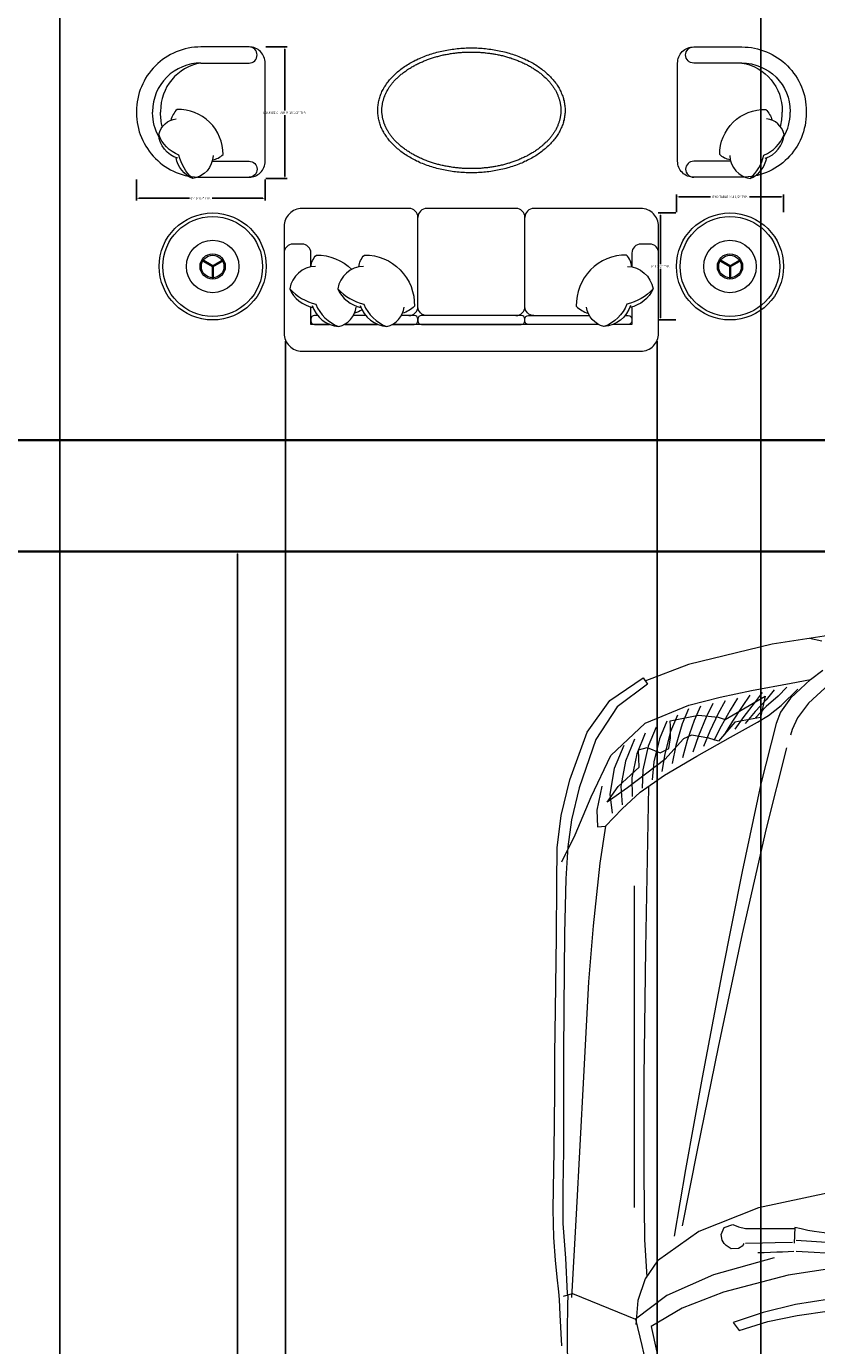
# Model space of a CAD drawing. Units: inches. Extents: x -36 to 401, y -686 to 73.
# Tile 7 of 15: x 184 to 248, y -485 to -379. Entities that reach past the tile are written whole.
import ezdxf

# ---------------------------------------------------------------- set-up
doc = ezdxf.new("R2010")
doc.units = ezdxf.units.IN
doc.header["$MEASUREMENT"] = 0
for name, color, linetype, lineweight in [('A-ANNO-DIMS', 2, 'Continuous', 18), ('A-FURN', 8, 'Continuous', 13), ('A-WALL', 7, 'Continuous', 35), ('C-PKNG-VEHI', 8, 'Continuous', 13)]:
    doc.layers.add(name, color=color, linetype=linetype, lineweight=lineweight)
doc.styles.get("Standard").update_dxf_attribs({"font": 'arial.ttf'})
doc.dimstyles.get("Standard").update_dxf_attribs({"dimtxt": 0.18, "dimasz": 0.18, "dimexe": 0.18, "dimexo": 0.0625, "dimgap": 0.09, "dimtad": 0, "dimtih": 1, "dimtoh": 1, "dimdec": 0, "dimzin": 0, "dimdsep": 46, "dimlunit": 3, "dimtxsty": 'Standard', "dimcen": 0.09, "dimadec": 0, "dimazin": 0, "dimtfac": 1, "dimtdec": 0, "dimtofl": 0, "dimtmove": 0, "dimatfit": 3, "dimfxl": 1, "dimtolj": 1, "dimtzin": 0, "dimarcsym": 0})

# ---------------------------------------------------------------- blocks, each defined once
blk = doc.blocks.new('*D3')
at = {"layer": 'A-ANNO-DIMS', "color": 0, "lineweight": -2, "transparency": 16777216}
for p, q in [((200.9, -421.21), (201.62, -421.21)), ((201.44, -421.39), (201.44, -532.06)), ((201.44, -649.03), (201.44, -538.36)), ((200.9, -649.21), (201.62, -649.21))]:
    blk.add_line(p, q, dxfattribs=at)
at = {"layer": 'A-ANNO-DIMS', "color": 0, "transparency": 16777216}
for points in [[(201.41, -421.39), (201.47, -421.39), (201.44, -421.21)], [(201.41, -649.03), (201.47, -649.03), (201.44, -649.21)]]:
    blk.add_solid(points, dxfattribs=at)
at = {"layer": 'Defpoints', "color": 0, "transparency": 16777216}
for p in [(200.84, -421.21), (200.84, -649.21), (201.44, -649.21)]:
    blk.add_point(p, dxfattribs=at)
at = {"layer": 'A-ANNO-DIMS', "color": 0, "transparency": 16777216, "insert": (201.44, -535.21), "char_height": 6, "attachment_point": 5}
blk.add_mtext("\\A1;19'", dxfattribs=at)
blk = doc.blocks.new('CHAIR-LOUNGE')
at = {"ltscale": 0.03}
blk.add_lwpolyline([(10.39, 5.37), (10.39, 9.33, 0.414214), (9.09, 10.63), (5.2, 10.63, 0.414214), (0, 5.43), (0, 5.37), (0, 5.3, 0.414214), (5.2, 0.11), (9.09, 0.11, 0.414214), (10.39, 1.4), (10.39, 5.37)], format="xyb", dxfattribs=at)
for points in [[(5.2, 9.33), (9.09, 9.33, 0.414214), (9.74, 9.98), (9.74, 9.98, 0.414214), (9.09, 10.63)], [(5.2, 9.33, 0.414214), (1.3, 5.43), (1.3, 5.37)], [(5.2, 9.33, 0.372719), (1.95, 5.43), (1.95, 5.37)], [(1.81, 3.37, -0.130591), (1.3, 5.3), (1.3, 5.37)], [(2.09, 4.19, -0.072384), (1.95, 5.3), (1.95, 5.37)], [(6.14, 1.53, 0.165541), (6.99, 1.94, 0.425989), (3.27, 5.58, 0.121523), (2.76, 4.72, -7.115464)], [(3.33, 1.64, -0.306663), (1.79, 3.57, -0.30633), (3.2, 4.84, 0.872847)], [(4.54, 0, -0.14773), (3.42, 1.9, -0.213343), (1.79, 3.57, -0.178662)], [(6.18, 1.86, -0.356772), (4.54, 0, -0.249542), (3.19, 1.69, 9.61688)], [(6.11, 1.4), (9.09, 1.4, -0.414214), (9.74, 0.76), (9.74, 0.76, -0.414214), (9.09, 0.11)]]:
    blk.add_lwpolyline(points, format="xyb")
blk = doc.blocks.new('END-TABLE-ROUND')
at = {"ltscale": 0.03}
for p, q in [((4.3, 4.28), (3.42, 4.79)), ((4.34, 4.36), (3.46, 4.87)), ((4.28, 4.32), (4.28, 3.31)), ((4.3, 4.36), (5.18, 4.87)), ((4.34, 4.28), (5.22, 4.79)), ((4.37, 4.32), (4.37, 3.31))]:
    blk.add_line(p, q, dxfattribs=at)
for radius in [4.32, 2.12, 1.02, 0.911]:
    blk.add_circle((4.32, 4.32), radius, dxfattribs=at)
blk.add_circle((4.32, 4.32), 4.03)
blk = doc.blocks.new('*D49')
at = {"layer": 'A-ANNO-DIMS', "color": 0, "lineweight": -2, "transparency": 16777216}
for p, q in [((203.74, -380.47), (205.45, -380.47)), ((205.27, -380.65), (205.27, -385.6)), ((205.27, -390.92), (205.27, -385.97)), ((203.74, -391.1), (205.45, -391.1))]:
    blk.add_line(p, q, dxfattribs=at)
at = {"layer": 'A-ANNO-DIMS', "color": 0, "transparency": 16777216}
for points in [[(205.24, -380.65), (205.3, -380.65), (205.27, -380.47)], [(205.24, -390.92), (205.3, -390.92), (205.27, -391.1)]]:
    blk.add_solid(points, dxfattribs=at)
at = {"layer": 'Defpoints', "color": 0, "transparency": 16777216}
for p in [(203.68, -380.47), (205.27, -380.47), (203.68, -391.1)]:
    blk.add_point(p, dxfattribs=at)
at = {"layer": 'A-ANNO-DIMS', "color": 0, "transparency": 16777216, "insert": (205.27, -385.78), "char_height": 0.18, "attachment_point": 5}
blk.add_mtext('\\A1;LOUNGE CHAIR 0\'-10 1/2" TYP.', dxfattribs=at)
blk = doc.blocks.new('*D50')
at = {"layer": 'A-ANNO-DIMS', "color": 0, "lineweight": -2, "transparency": 16777216}
for p, q in [((193.29, -391.16), (193.29, -392.87)), ((203.68, -391.16), (203.68, -392.87)), ((193.47, -392.69), (197.56, -392.69)), ((203.5, -392.69), (199.4, -392.69))]:
    blk.add_line(p, q, dxfattribs=at)
at = {"layer": 'A-ANNO-DIMS', "color": 0, "transparency": 16777216}
for points in [[(193.47, -392.66), (193.47, -392.72), (193.29, -392.69)], [(203.5, -392.66), (203.5, -392.72), (203.68, -392.69)]]:
    blk.add_solid(points, dxfattribs=at)
at = {"layer": 'Defpoints', "color": 0, "transparency": 16777216}
for p in [(193.29, -391.1), (203.68, -391.1), (203.68, -392.69)]:
    blk.add_point(p, dxfattribs=at)
at = {"layer": 'A-ANNO-DIMS', "color": 0, "transparency": 16777216, "insert": (198.48, -392.69), "char_height": 0.18, "attachment_point": 5}
blk.add_mtext('\\A1;0\'-10 1/2" TYP.', dxfattribs=at)
blk = doc.blocks.new('*D51')
at = {"layer": 'A-ANNO-DIMS', "color": 0, "lineweight": -2, "transparency": 16777216}
for p, q in [((236.89, -393.81), (236.89, -392.39)), ((237.07, -392.57), (239.64, -392.57)), ((245.36, -392.57), (242.79, -392.57)), ((245.54, -393.81), (245.54, -392.39))]:
    blk.add_line(p, q, dxfattribs=at)
at = {"layer": 'A-ANNO-DIMS', "color": 0, "transparency": 16777216}
for points in [[(237.07, -392.54), (237.07, -392.6), (236.89, -392.57)], [(245.36, -392.54), (245.36, -392.6), (245.54, -392.57)]]:
    blk.add_solid(points, dxfattribs=at)
at = {"layer": 'Defpoints', "color": 0, "transparency": 16777216}
for p in [(245.54, -392.57), (236.89, -393.87), (245.54, -393.87)]:
    blk.add_point(p, dxfattribs=at)
at = {"layer": 'A-ANNO-DIMS', "color": 0, "transparency": 16777216, "insert": (241.22, -392.57), "char_height": 0.18, "attachment_point": 5}
blk.add_mtext('\\A1;END TABLE 0\'-8 1/2" TYP.', dxfattribs=at)
blk = doc.blocks.new('*D52')
at = {"layer": 'A-ANNO-DIMS', "color": 0, "lineweight": -2, "transparency": 16777216}
for p, q in [((236.83, -393.87), (235.42, -393.87)), ((235.6, -394.05), (235.6, -398.01)), ((235.6, -402.33), (235.6, -398.37)), ((236.83, -402.51), (235.42, -402.51))]:
    blk.add_line(p, q, dxfattribs=at)
at = {"layer": 'A-ANNO-DIMS', "color": 0, "transparency": 16777216}
for points in [[(235.57, -394.05), (235.63, -394.05), (235.6, -393.87)], [(235.57, -402.33), (235.63, -402.33), (235.6, -402.51)]]:
    blk.add_solid(points, dxfattribs=at)
at = {"layer": 'Defpoints', "color": 0, "transparency": 16777216}
for p in [(235.6, -393.87), (236.89, -393.87), (236.89, -402.51)]:
    blk.add_point(p, dxfattribs=at)
at = {"layer": 'A-ANNO-DIMS', "color": 0, "transparency": 16777216, "insert": (235.6, -398.19), "char_height": 0.18, "attachment_point": 5}
blk.add_mtext('\\A1;0\'-8 1/2" TYP.', dxfattribs=at)
blk = doc.blocks.new('*D73')
at = {"layer": 'A-ANNO-DIMS', "color": 0, "lineweight": -2, "transparency": 16777216}
for p, q in [((177.19, -421.27), (177.19, -685.69)), ((253.69, -421.27), (253.69, -685.69)), ((177.37, -685.51), (214.9, -685.51)), ((253.51, -685.51), (215.98, -685.51))]:
    blk.add_line(p, q, dxfattribs=at)
at = {"layer": 'A-ANNO-DIMS', "color": 0, "transparency": 16777216}
for points in [[(177.37, -685.48), (177.37, -685.54), (177.19, -685.51)], [(253.51, -685.48), (253.51, -685.54), (253.69, -685.51)]]:
    blk.add_solid(points, dxfattribs=at)
at = {"layer": 'Defpoints', "color": 0, "transparency": 16777216}
for p in [(177.19, -421.21), (253.69, -421.21), (253.69, -685.51)]:
    blk.add_point(p, dxfattribs=at)
at = {"layer": 'A-ANNO-DIMS', "color": 0, "transparency": 16777216, "insert": (215.44, -685.51), "char_height": 0.18, "attachment_point": 5}
blk.add_mtext('\\A1;6\'-4 1/2"', dxfattribs=at)
blk = doc.blocks.new('*D87')
at = {"layer": 'A-ANNO-DIMS', "color": 0, "lineweight": -2, "transparency": 16777216}
for p, q in [((243.7, -154.81), (243.7, -685.69)), ((187.11, -163.6), (187.11, -685.69)), ((187.29, -685.51), (214.86, -685.51)), ((243.52, -685.51), (215.95, -685.51))]:
    blk.add_line(p, q, dxfattribs=at)
at = {"layer": 'A-ANNO-DIMS', "color": 0, "transparency": 16777216}
for points in [[(187.29, -685.48), (187.29, -685.54), (187.11, -685.51)], [(243.52, -685.48), (243.52, -685.54), (243.7, -685.51)]]:
    blk.add_solid(points, dxfattribs=at)
at = {"layer": 'Defpoints', "color": 0, "transparency": 16777216}
for p in [(243.7, -154.75), (187.11, -163.53), (243.7, -685.51)]:
    blk.add_point(p, dxfattribs=at)
at = {"layer": 'A-ANNO-DIMS', "color": 0, "transparency": 16777216, "insert": (215.4, -685.51), "char_height": 0.18, "attachment_point": 5}
blk.add_mtext('\\A1;4\'-8 1/2"', dxfattribs=at)
blk = doc.blocks.new('*D91')
at = {"layer": 'A-ANNO-DIMS', "color": 0, "lineweight": -2, "transparency": 16777216}
for p, q in [((205.32, -404.21), (205.32, -685.69)), ((235.34, -404.21), (235.34, -685.69)), ((205.5, -685.51), (220, -685.51)), ((235.16, -685.51), (220.66, -685.51))]:
    blk.add_line(p, q, dxfattribs=at)
at = {"layer": 'A-ANNO-DIMS', "color": 0, "transparency": 16777216}
for points in [[(205.5, -685.48), (205.5, -685.54), (205.32, -685.51)], [(235.16, -685.48), (235.16, -685.54), (235.34, -685.51)]]:
    blk.add_solid(points, dxfattribs=at)
at = {"layer": 'Defpoints', "color": 0, "transparency": 16777216}
for p in [(205.32, -404.14), (235.34, -404.14), (235.34, -685.51)]:
    blk.add_point(p, dxfattribs=at)
at = {"layer": 'A-ANNO-DIMS', "color": 0, "transparency": 16777216, "insert": (220.33, -685.51), "char_height": 0.18, "attachment_point": 5}
blk.add_mtext('\\A1;2\'-6"', dxfattribs=at)

msp = doc.modelspace()

# ---------------------------------------------------------------- linework, layer by layer
at = {"layer": 'A-FURN', "ltscale": 0.03}
msp.add_lwpolyline([(235.45, -394.95, 0.414214), (234.01, -393.51), (225.37, -393.51, 0.414214), (224.65, -394.23, 0.414214), (223.93, -393.51), (216.73, -393.51, 0.414214), (216.01, -394.23, 0.414214), (215.29, -393.51), (206.65, -393.51, 0.414214), (205.21, -394.95), (205.21, -403.59, 0.414214), (206.65, -405.03), (234.01, -405.03, 0.414214), (235.45, -403.59)], format="xyb", close=True, dxfattribs=at)
at = {"layer": 'A-FURN'}
for points in [[(215.29, -402.15, 0.414214), (216.01, -401.43), (216.01, -394.23, 0.414214)], [(225.37, -402.15, -0.414214), (224.65, -401.43), (224.65, -394.23, -0.414214)], [(207.37, -398.23), (207.37, -397.11, 0.414214), (206.65, -396.39), (205.93, -396.39, 0.414214), (205.21, -397.11)], [(235.45, -397.11, 0.414214), (234.73, -396.39), (234.01, -396.39, 0.414214), (233.29, -397.11), (233.29, -398.23)], [(207.73, -398.18, 0.356772), (205.66, -400, 0.249542), (207.53, -401.49, -9.61688)], [(207.36, -398.23, -0.165541), (207.81, -397.27, -0.200231), (210.67, -398.43, -0.121523)], [(211.61, -398.18, 0.356772), (209.54, -400, 0.249542), (211.41, -401.49, -9.61688)], [(211.24, -398.23, -0.165541), (211.69, -397.27, -0.425989), (215.73, -401.4, -0.121523), (214.77, -401.97, 7.115464)], [(233.29, -398.23, 0.165541), (232.85, -397.27, 0.425989), (228.8, -401.4, 0.121523), (229.76, -401.97, -7.115464)], [(232.93, -398.18, -0.356772), (235, -400, -0.249542), (233.13, -401.49, 9.61688)], [(205.66, -400, 0.14773), (207.77, -401.24, 0.213343), (209.63, -403.05, 0.178662)], [(209.54, -400, 0.14773), (211.65, -401.24, 0.213343), (213.51, -403.05, 0.178662)], [(235, -400, -0.14773), (232.89, -401.24, -0.213343), (231.03, -403.05, -0.178662)], [(208.88, -402.87), (207.37, -402.87), (207.37, -401.46, 0.414214)], [(207.48, -401.33, 0.306663), (209.63, -403.05, 0.30633), (211.03, -401.48, -0.872847)], [(211.36, -401.33, 0.306663), (213.51, -403.05, 0.30633), (214.91, -401.48, -0.872847)], [(216.73, -402.15, -0.414214), (216.01, -401.43)], [(223.93, -402.15, 0.414214), (224.65, -401.43)], [(233.18, -401.33, -0.306663), (231.03, -403.05, -0.30633), (229.63, -401.48, 0.872847)], [(207.92, -402.15), (207.65, -402.15, 0.414214), (207.37, -402.44), (207.37, -402.58, 0.414214), (207.65, -402.87)], [(211.8, -402.15), (210.8, -402.15, 0.414214)], [(211.5, -401.69, -0.071865), (210.89, -401.97, 7.115464)], [(213.96, -402.87), (215.72, -402.87, 0.414214), (216.01, -402.58), (216.01, -402.44, 0.414214), (215.72, -402.15), (214.68, -402.15, 0.414214)], [(230.58, -402.87), (224.94, -402.87, -0.414214), (224.65, -402.58), (224.65, -402.44, -0.414214), (224.94, -402.15), (229.85, -402.15, -0.414214)], [(232.74, -402.15), (233, -402.15, -0.414214), (233.29, -402.44), (233.29, -402.58, -0.414214), (233, -402.87)], [(207.65, -402.87), (208.88, -402.87, 0.414214)], [(210.08, -402.87), (212.76, -402.87, 0.414214)], [(233, -402.87), (231.78, -402.87, -0.414214)]]:
    msp.add_lwpolyline(points, format="xyb", dxfattribs=at)
for points in [[(233.29, -401.46), (233.29, -402.87), (231.78, -402.87)], [(212.76, -402.87), (210.08, -402.87)], [(230.58, -402.87), (213.96, -402.87)]]:
    msp.add_lwpolyline(points, dxfattribs=at)
msp.add_lwpolyline([(216.3, -402.87), (224.36, -402.87, 0.414214), (224.65, -402.58), (224.65, -402.44, 0.414214), (224.36, -402.15), (216.3, -402.15, 0.414214), (216.01, -402.44), (216.01, -402.58, 0.414214)], format="xyb", close=True, dxfattribs=at)
at = {"layer": 'A-FURN', "ltscale": 0.03}
msp.add_polyline3d([(227.89, -385.59, 0), (227.89, -385.68, 0), (227.89, -385.78, 0), (227.88, -385.87, 0), (227.87, -385.97, 0), (227.86, -386.06, 0), (227.84, -386.16, 0), (227.83, -386.25, 0), (227.81, -386.35, 0), (227.78, -386.44, 0), (227.76, -386.54, 0), (227.73, -386.63, 0), (227.7, -386.72, 0), (227.66, -386.81, 0), (227.63, -386.91, 0), (227.59, -387, 0), (227.55, -387.09, 0), (227.5, -387.18, 0), (227.46, -387.27, 0), (227.41, -387.36, 0), (227.36, -387.45, 0), (227.3, -387.54, 0), (227.25, -387.63, 0), (227.19, -387.71, 0), (227.12, -387.8, 0), (227.06, -387.88, 0), (226.99, -387.97, 0), (226.93, -388.05, 0), (226.85, -388.14, 0), (226.78, -388.22, 0), (226.71, -388.3, 0), (226.63, -388.38, 0), (226.55, -388.46, 0), (226.46, -388.53, 0), (226.38, -388.61, 0), (226.29, -388.69, 0), (226.2, -388.76, 0), (226.11, -388.84, 0), (226.02, -388.91, 0), (225.92, -388.98, 0), (225.83, -389.05, 0), (225.73, -389.12, 0), (225.63, -389.19, 0), (225.52, -389.25, 0), (225.42, -389.32, 0), (225.31, -389.38, 0), (225.2, -389.44, 0), (225.09, -389.5, 0), (224.98, -389.56, 0), (224.87, -389.62, 0), (224.75, -389.68, 0), (224.63, -389.73, 0), (224.52, -389.79, 0), (224.4, -389.84, 0), (224.27, -389.89, 0), (224.15, -389.94, 0), (224.03, -389.98, 0), (223.9, -390.03, 0), (223.78, -390.07, 0), (223.65, -390.12, 0), (223.52, -390.16, 0), (223.39, -390.2, 0), (223.26, -390.24, 0), (223.12, -390.27, 0), (222.99, -390.31, 0), (222.86, -390.34, 0), (222.72, -390.37, 0), (222.58, -390.4, 0), (222.45, -390.43, 0), (222.31, -390.45, 0), (222.17, -390.48, 0), (222.03, -390.5, 0), (221.89, -390.52, 0), (221.75, -390.54, 0), (221.61, -390.56, 0), (221.47, -390.57, 0), (221.33, -390.58, 0), (221.19, -390.6, 0), (221.04, -390.61, 0), (220.9, -390.61, 0), (220.76, -390.62, 0), (220.62, -390.62, 0), (220.47, -390.63, 0), (220.33, -390.63, 0), (220.19, -390.63, 0), (220.04, -390.62, 0), (219.9, -390.62, 0), (219.76, -390.61, 0), (219.62, -390.61, 0), (219.47, -390.6, 0), (219.33, -390.58, 0), (219.19, -390.57, 0), (219.05, -390.56, 0), (218.91, -390.54, 0), (218.77, -390.52, 0), (218.63, -390.5, 0), (218.49, -390.48, 0), (218.35, -390.45, 0), (218.21, -390.43, 0), (218.07, -390.4, 0), (217.94, -390.37, 0), (217.8, -390.34, 0), (217.67, -390.31, 0), (217.54, -390.27, 0), (217.4, -390.24, 0), (217.27, -390.2, 0), (217.14, -390.16, 0), (217.01, -390.12, 0), (216.88, -390.07, 0), (216.76, -390.03, 0), (216.63, -389.98, 0), (216.51, -389.94, 0), (216.38, -389.89, 0), (216.26, -389.84, 0), (216.14, -389.79, 0), (216.02, -389.73, 0), (215.91, -389.68, 0), (215.79, -389.62, 0), (215.68, -389.56, 0), (215.57, -389.5, 0), (215.46, -389.44, 0), (215.35, -389.38, 0), (215.24, -389.32, 0), (215.14, -389.25, 0), (215.03, -389.19, 0), (214.93, -389.12, 0), (214.83, -389.05, 0), (214.74, -388.98, 0), (214.64, -388.91, 0), (214.55, -388.84, 0), (214.46, -388.76, 0), (214.37, -388.69, 0), (214.28, -388.61, 0), (214.2, -388.53, 0), (214.11, -388.46, 0), (214.03, -388.38, 0), (213.95, -388.3, 0), (213.88, -388.22, 0), (213.8, -388.14, 0), (213.73, -388.05, 0), (213.66, -387.97, 0), (213.6, -387.88, 0), (213.53, -387.8, 0), (213.47, -387.71, 0), (213.41, -387.63, 0), (213.36, -387.54, 0), (213.3, -387.45, 0), (213.25, -387.36, 0), (213.2, -387.27, 0), (213.16, -387.18, 0), (213.11, -387.09, 0), (213.07, -387, 0), (213.03, -386.91, 0), (213, -386.81, 0), (212.96, -386.72, 0), (212.93, -386.63, 0), (212.9, -386.54, 0), (212.88, -386.44, 0), (212.85, -386.35, 0), (212.83, -386.25, 0), (212.82, -386.16, 0), (212.8, -386.06, 0), (212.79, -385.97, 0), (212.78, -385.87, 0), (212.77, -385.78, 0), (212.77, -385.68, 0), (212.77, -385.59, 0), (212.77, -385.49, 0), (212.77, -385.4, 0), (212.78, -385.3, 0), (212.79, -385.21, 0), (212.8, -385.11, 0), (212.82, -385.02, 0), (212.83, -384.92, 0), (212.85, -384.83, 0), (212.88, -384.73, 0), (212.9, -384.64, 0), (212.93, -384.55, 0), (212.96, -384.45, 0), (213, -384.36, 0), (213.03, -384.27, 0), (213.07, -384.18, 0), (213.11, -384.08, 0), (213.16, -383.99, 0), (213.2, -383.9, 0), (213.25, -383.81, 0), (213.3, -383.72, 0), (213.36, -383.64, 0), (213.41, -383.55, 0), (213.47, -383.46, 0), (213.53, -383.38, 0), (213.6, -383.29, 0), (213.66, -383.21, 0), (213.73, -383.12, 0), (213.8, -383.04, 0), (213.88, -382.96, 0), (213.95, -382.88, 0), (214.03, -382.8, 0), (214.11, -382.72, 0), (214.2, -382.64, 0), (214.28, -382.56, 0), (214.37, -382.49, 0), (214.46, -382.41, 0), (214.55, -382.34, 0), (214.64, -382.27, 0), (214.74, -382.19, 0), (214.83, -382.12, 0), (214.93, -382.06, 0), (215.03, -381.99, 0), (215.14, -381.92, 0), (215.24, -381.86, 0), (215.35, -381.79, 0), (215.46, -381.73, 0), (215.57, -381.67, 0), (215.68, -381.61, 0), (215.79, -381.55, 0), (215.91, -381.5, 0), (216.02, -381.44, 0), (216.14, -381.39, 0), (216.26, -381.34, 0), (216.38, -381.29, 0), (216.51, -381.24, 0), (216.63, -381.19, 0), (216.76, -381.14, 0), (216.88, -381.1, 0), (217.01, -381.06, 0), (217.14, -381.02, 0), (217.27, -380.98, 0), (217.4, -380.94, 0), (217.54, -380.9, 0), (217.67, -380.87, 0), (217.8, -380.84, 0), (217.94, -380.8, 0), (218.07, -380.78, 0), (218.21, -380.75, 0), (218.35, -380.72, 0), (218.49, -380.7, 0), (218.63, -380.68, 0), (218.77, -380.65, 0), (218.91, -380.64, 0), (219.05, -380.62, 0), (219.19, -380.6, 0), (219.33, -380.59, 0), (219.47, -380.58, 0), (219.62, -380.57, 0), (219.76, -380.56, 0), (219.9, -380.55, 0), (220.04, -380.55, 0), (220.19, -380.55, 0), (220.33, -380.55, 0), (220.47, -380.55, 0), (220.62, -380.55, 0), (220.76, -380.55, 0), (220.9, -380.56, 0), (221.04, -380.57, 0), (221.19, -380.58, 0), (221.33, -380.59, 0), (221.47, -380.6, 0), (221.61, -380.62, 0), (221.75, -380.64, 0), (221.89, -380.65, 0), (222.03, -380.68, 0), (222.17, -380.7, 0), (222.31, -380.72, 0), (222.45, -380.75, 0), (222.58, -380.78, 0), (222.72, -380.8, 0), (222.86, -380.84, 0), (222.99, -380.87, 0), (223.12, -380.9, 0), (223.26, -380.94, 0), (223.39, -380.98, 0), (223.52, -381.02, 0), (223.65, -381.06, 0), (223.78, -381.1, 0), (223.9, -381.14, 0), (224.03, -381.19, 0), (224.15, -381.24, 0), (224.27, -381.29, 0), (224.4, -381.34, 0), (224.52, -381.39, 0), (224.63, -381.44, 0), (224.75, -381.5, 0), (224.87, -381.55, 0), (224.98, -381.61, 0), (225.09, -381.67, 0), (225.2, -381.73, 0), (225.31, -381.79, 0), (225.42, -381.86, 0), (225.52, -381.92, 0), (225.63, -381.99, 0), (225.73, -382.06, 0), (225.83, -382.12, 0), (225.92, -382.19, 0), (226.02, -382.27, 0), (226.11, -382.34, 0), (226.2, -382.41, 0), (226.29, -382.49, 0), (226.38, -382.56, 0), (226.46, -382.64, 0), (226.55, -382.72, 0), (226.63, -382.8, 0), (226.71, -382.88, 0), (226.78, -382.96, 0), (226.85, -383.04, 0), (226.93, -383.12, 0), (226.99, -383.21, 0), (227.06, -383.29, 0), (227.12, -383.38, 0), (227.19, -383.46, 0), (227.25, -383.55, 0), (227.3, -383.64, 0), (227.36, -383.72, 0), (227.41, -383.81, 0), (227.46, -383.9, 0), (227.5, -383.99, 0), (227.55, -384.08, 0), (227.59, -384.18, 0), (227.63, -384.27, 0), (227.66, -384.36, 0), (227.7, -384.45, 0), (227.73, -384.55, 0), (227.76, -384.64, 0), (227.78, -384.73, 0), (227.81, -384.83, 0), (227.83, -384.92, 0), (227.84, -385.02, 0), (227.86, -385.11, 0), (227.87, -385.21, 0), (227.88, -385.3, 0), (227.89, -385.4, 0), (227.89, -385.49, 0), (227.89, -385.59, 0)], dxfattribs=at)
at = {"layer": 'A-FURN'}
msp.add_polyline3d([(227.56, -385.59, 0), (227.56, -385.64, 0), (227.55, -385.69, 0), (227.55, -385.74, 0), (227.55, -385.79, 0), (227.54, -385.85, 0), (227.54, -385.9, 0), (227.53, -385.95, 0), (227.53, -386.01, 0), (227.52, -386.06, 0), (227.51, -386.11, 0), (227.5, -386.17, 0), (227.49, -386.22, 0), (227.48, -386.27, 0), (227.46, -386.33, 0), (227.45, -386.38, 0), (227.44, -386.44, 0), (227.42, -386.49, 0), (227.4, -386.55, 0), (227.38, -386.6, 0), (227.36, -386.66, 0), (227.34, -386.71, 0), (227.32, -386.77, 0), (227.3, -386.82, 0), (227.28, -386.88, 0), (227.25, -386.93, 0), (227.22, -386.99, 0), (227.2, -387.04, 0), (227.17, -387.1, 0), (227.14, -387.15, 0), (227.11, -387.21, 0), (227.08, -387.26, 0), (227.04, -387.32, 0), (227.01, -387.37, 0), (226.97, -387.43, 0), (226.94, -387.48, 0), (226.9, -387.54, 0), (226.86, -387.59, 0), (226.82, -387.64, 0), (226.78, -387.7, 0), (226.74, -387.75, 0), (226.69, -387.81, 0), (226.65, -387.86, 0), (226.6, -387.91, 0), (226.56, -387.96, 0), (226.51, -388.02, 0), (226.46, -388.07, 0), (226.41, -388.12, 0), (226.36, -388.17, 0), (226.3, -388.22, 0), (226.25, -388.27, 0), (226.19, -388.32, 0), (226.14, -388.37, 0), (226.08, -388.42, 0), (226.02, -388.47, 0), (225.96, -388.52, 0), (225.9, -388.57, 0), (225.84, -388.62, 0), (225.77, -388.67, 0), (225.71, -388.71, 0), (225.64, -388.76, 0), (225.58, -388.81, 0), (225.51, -388.85, 0), (225.44, -388.9, 0), (225.38, -388.94, 0), (225.31, -388.99, 0), (225.24, -389.03, 0), (225.16, -389.07, 0), (225.09, -389.11, 0), (225.02, -389.15, 0), (224.95, -389.2, 0), (224.87, -389.24, 0), (224.8, -389.28, 0), (224.72, -389.31, 0), (224.64, -389.35, 0), (224.57, -389.39, 0), (224.49, -389.43, 0), (224.41, -389.46, 0), (224.33, -389.5, 0), (224.25, -389.53, 0), (224.17, -389.57, 0), (224.09, -389.6, 0), (224.01, -389.63, 0), (223.92, -389.66, 0), (223.84, -389.7, 0), (223.76, -389.72, 0), (223.67, -389.75, 0), (223.59, -389.78, 0), (223.51, -389.81, 0), (223.42, -389.84, 0), (223.34, -389.86, 0), (223.25, -389.89, 0), (223.17, -389.91, 0), (223.09, -389.93, 0), (223, -389.96, 0), (222.92, -389.98, 0), (222.83, -390, 0), (222.74, -390.02, 0), (222.66, -390.04, 0), (222.57, -390.06, 0), (222.49, -390.08, 0), (222.4, -390.09, 0), (222.31, -390.11, 0), (222.23, -390.13, 0), (222.14, -390.14, 0), (222.06, -390.16, 0), (221.97, -390.17, 0), (221.88, -390.18, 0), (221.79, -390.2, 0), (221.71, -390.21, 0), (221.62, -390.22, 0), (221.53, -390.23, 0), (221.45, -390.24, 0), (221.36, -390.24, 0), (221.27, -390.25, 0), (221.18, -390.26, 0), (221.1, -390.27, 0), (221.01, -390.27, 0), (220.92, -390.28, 0), (220.83, -390.28, 0), (220.75, -390.28, 0), (220.66, -390.29, 0), (220.57, -390.29, 0), (220.48, -390.29, 0), (220.4, -390.29, 0), (220.31, -390.29, 0), (220.22, -390.29, 0), (220.13, -390.29, 0), (220.04, -390.29, 0), (219.96, -390.29, 0), (219.87, -390.28, 0), (219.78, -390.28, 0), (219.69, -390.27, 0), (219.61, -390.27, 0), (219.52, -390.26, 0), (219.43, -390.26, 0), (219.34, -390.25, 0), (219.26, -390.24, 0), (219.17, -390.23, 0), (219.08, -390.22, 0), (218.99, -390.21, 0), (218.91, -390.2, 0), (218.82, -390.19, 0), (218.73, -390.18, 0), (218.65, -390.16, 0), (218.56, -390.15, 0), (218.47, -390.13, 0), (218.39, -390.12, 0), (218.3, -390.1, 0), (218.22, -390.09, 0), (218.13, -390.07, 0), (218.04, -390.05, 0), (217.96, -390.03, 0), (217.87, -390.01, 0), (217.79, -389.99, 0), (217.7, -389.97, 0), (217.62, -389.95, 0), (217.53, -389.92, 0), (217.45, -389.9, 0), (217.36, -389.87, 0), (217.28, -389.85, 0), (217.19, -389.82, 0), (217.11, -389.8, 0), (217.03, -389.77, 0), (216.94, -389.74, 0), (216.86, -389.71, 0), (216.78, -389.68, 0), (216.69, -389.65, 0), (216.61, -389.62, 0), (216.53, -389.58, 0), (216.45, -389.55, 0), (216.37, -389.52, 0), (216.29, -389.48, 0), (216.21, -389.45, 0), (216.13, -389.41, 0), (216.05, -389.37, 0), (215.98, -389.33, 0), (215.9, -389.3, 0), (215.83, -389.26, 0), (215.75, -389.22, 0), (215.68, -389.18, 0), (215.6, -389.13, 0), (215.53, -389.09, 0), (215.46, -389.05, 0), (215.39, -389.01, 0), (215.32, -388.96, 0), (215.25, -388.92, 0), (215.18, -388.87, 0), (215.11, -388.83, 0), (215.05, -388.78, 0), (214.98, -388.74, 0), (214.92, -388.69, 0), (214.85, -388.64, 0), (214.79, -388.6, 0), (214.73, -388.55, 0), (214.67, -388.5, 0), (214.61, -388.45, 0), (214.55, -388.4, 0), (214.5, -388.35, 0), (214.44, -388.3, 0), (214.38, -388.25, 0), (214.33, -388.2, 0), (214.28, -388.15, 0), (214.23, -388.09, 0), (214.18, -388.04, 0), (214.13, -387.99, 0), (214.08, -387.94, 0), (214.03, -387.88, 0), (213.99, -387.83, 0), (213.94, -387.78, 0), (213.9, -387.72, 0), (213.86, -387.67, 0), (213.82, -387.62, 0), (213.78, -387.56, 0), (213.74, -387.51, 0), (213.7, -387.45, 0), (213.67, -387.4, 0), (213.63, -387.34, 0), (213.6, -387.29, 0), (213.57, -387.23, 0), (213.53, -387.18, 0), (213.5, -387.12, 0), (213.48, -387.07, 0), (213.45, -387.01, 0), (213.42, -386.96, 0), (213.4, -386.9, 0), (213.37, -386.85, 0), (213.35, -386.79, 0), (213.33, -386.74, 0), (213.3, -386.68, 0), (213.28, -386.63, 0), (213.27, -386.57, 0), (213.25, -386.52, 0), (213.23, -386.46, 0), (213.22, -386.41, 0), (213.2, -386.35, 0), (213.19, -386.3, 0), (213.18, -386.25, 0), (213.16, -386.19, 0), (213.15, -386.14, 0), (213.14, -386.09, 0), (213.14, -386.03, 0), (213.13, -385.98, 0), (213.12, -385.93, 0), (213.12, -385.87, 0), (213.11, -385.82, 0), (213.11, -385.77, 0), (213.11, -385.72, 0), (213.1, -385.66, 0), (213.1, -385.61, 0), (213.1, -385.56, 0), (213.1, -385.51, 0), (213.11, -385.46, 0), (213.11, -385.41, 0), (213.11, -385.35, 0), (213.12, -385.3, 0), (213.12, -385.25, 0), (213.13, -385.19, 0), (213.14, -385.14, 0), (213.14, -385.09, 0), (213.15, -385.03, 0), (213.16, -384.98, 0), (213.18, -384.93, 0), (213.19, -384.87, 0), (213.2, -384.82, 0), (213.22, -384.76, 0), (213.23, -384.71, 0), (213.25, -384.66, 0), (213.27, -384.6, 0), (213.28, -384.55, 0), (213.3, -384.49, 0), (213.33, -384.44, 0), (213.35, -384.38, 0), (213.37, -384.33, 0), (213.4, -384.27, 0), (213.42, -384.22, 0), (213.45, -384.16, 0), (213.48, -384.11, 0), (213.5, -384.05, 0), (213.53, -384, 0), (213.57, -383.94, 0), (213.6, -383.88, 0), (213.63, -383.83, 0), (213.67, -383.78, 0), (213.7, -383.72, 0), (213.74, -383.67, 0), (213.78, -383.61, 0), (213.82, -383.56, 0), (213.86, -383.5, 0), (213.9, -383.45, 0), (213.94, -383.4, 0), (213.99, -383.34, 0), (214.03, -383.29, 0), (214.08, -383.24, 0), (214.13, -383.18, 0), (214.18, -383.13, 0), (214.23, -383.08, 0), (214.28, -383.03, 0), (214.33, -382.98, 0), (214.38, -382.93, 0), (214.44, -382.87, 0), (214.5, -382.82, 0), (214.55, -382.77, 0), (214.61, -382.72, 0), (214.67, -382.68, 0), (214.73, -382.63, 0), (214.79, -382.58, 0), (214.85, -382.53, 0), (214.92, -382.48, 0), (214.98, -382.44, 0), (215.05, -382.39, 0), (215.11, -382.34, 0), (215.18, -382.3, 0), (215.25, -382.25, 0), (215.32, -382.21, 0), (215.39, -382.17, 0), (215.46, -382.12, 0), (215.53, -382.08, 0), (215.6, -382.04, 0), (215.68, -382, 0), (215.75, -381.96, 0), (215.83, -381.92, 0), (215.9, -381.88, 0), (215.98, -381.84, 0), (216.05, -381.8, 0), (216.13, -381.76, 0), (216.21, -381.73, 0), (216.29, -381.69, 0), (216.37, -381.66, 0), (216.45, -381.62, 0), (216.53, -381.59, 0), (216.61, -381.56, 0), (216.69, -381.53, 0), (216.78, -381.49, 0), (216.86, -381.46, 0), (216.94, -381.43, 0), (217.03, -381.41, 0), (217.11, -381.38, 0), (217.19, -381.35, 0), (217.28, -381.32, 0), (217.36, -381.3, 0), (217.45, -381.27, 0), (217.53, -381.25, 0), (217.62, -381.23, 0), (217.7, -381.21, 0), (217.79, -381.18, 0), (217.87, -381.16, 0), (217.96, -381.14, 0), (218.04, -381.12, 0), (218.13, -381.11, 0), (218.22, -381.09, 0), (218.3, -381.07, 0), (218.39, -381.05, 0), (218.47, -381.04, 0), (218.56, -381.02, 0), (218.65, -381.01, 0), (218.73, -381, 0), (218.82, -380.98, 0), (218.91, -380.97, 0), (218.99, -380.96, 0), (219.08, -380.95, 0), (219.17, -380.94, 0), (219.26, -380.93, 0), (219.34, -380.93, 0), (219.43, -380.92, 0), (219.52, -380.91, 0), (219.61, -380.9, 0), (219.69, -380.9, 0), (219.78, -380.9, 0), (219.87, -380.89, 0), (219.96, -380.89, 0), (220.04, -380.89, 0), (220.13, -380.88, 0), (220.22, -380.88, 0), (220.31, -380.88, 0), (220.4, -380.88, 0), (220.48, -380.88, 0), (220.57, -380.88, 0), (220.66, -380.89, 0), (220.75, -380.89, 0), (220.83, -380.89, 0), (220.92, -380.9, 0), (221.01, -380.9, 0), (221.1, -380.91, 0), (221.18, -380.91, 0), (221.27, -380.92, 0), (221.36, -380.93, 0), (221.45, -380.94, 0), (221.53, -380.95, 0), (221.62, -380.96, 0), (221.71, -380.97, 0), (221.79, -380.98, 0), (221.88, -380.99, 0), (221.97, -381, 0), (222.06, -381.02, 0), (222.14, -381.03, 0), (222.23, -381.05, 0), (222.31, -381.06, 0), (222.4, -381.08, 0), (222.49, -381.1, 0), (222.57, -381.11, 0), (222.66, -381.13, 0), (222.74, -381.15, 0), (222.83, -381.17, 0), (222.92, -381.19, 0), (223, -381.22, 0), (223.09, -381.24, 0), (223.17, -381.26, 0), (223.25, -381.29, 0), (223.34, -381.31, 0), (223.42, -381.34, 0), (223.51, -381.36, 0), (223.59, -381.39, 0), (223.67, -381.42, 0), (223.76, -381.45, 0), (223.84, -381.48, 0), (223.92, -381.51, 0), (224.01, -381.54, 0), (224.09, -381.57, 0), (224.17, -381.61, 0), (224.25, -381.64, 0), (224.33, -381.68, 0), (224.41, -381.71, 0), (224.49, -381.75, 0), (224.57, -381.78, 0), (224.64, -381.82, 0), (224.72, -381.86, 0), (224.8, -381.9, 0), (224.87, -381.94, 0), (224.95, -381.98, 0), (225.02, -382.02, 0), (225.09, -382.06, 0), (225.16, -382.1, 0), (225.24, -382.15, 0), (225.31, -382.19, 0), (225.38, -382.23, 0), (225.44, -382.28, 0), (225.51, -382.32, 0), (225.58, -382.37, 0), (225.64, -382.41, 0), (225.71, -382.46, 0), (225.77, -382.51, 0), (225.84, -382.56, 0), (225.9, -382.6, 0), (225.96, -382.65, 0), (226.02, -382.7, 0), (226.08, -382.75, 0), (226.14, -382.8, 0), (226.19, -382.85, 0), (226.25, -382.9, 0), (226.3, -382.95, 0), (226.36, -383, 0), (226.41, -383.05, 0), (226.46, -383.11, 0), (226.51, -383.16, 0), (226.56, -383.21, 0), (226.6, -383.26, 0), (226.65, -383.32, 0), (226.69, -383.37, 0), (226.74, -383.42, 0), (226.78, -383.48, 0), (226.82, -383.53, 0), (226.86, -383.58, 0), (226.9, -383.64, 0), (226.94, -383.69, 0), (226.97, -383.75, 0), (227.01, -383.8, 0), (227.04, -383.86, 0), (227.08, -383.91, 0), (227.11, -383.97, 0), (227.14, -384.02, 0), (227.17, -384.08, 0), (227.2, -384.13, 0), (227.22, -384.19, 0), (227.25, -384.24, 0), (227.28, -384.3, 0), (227.3, -384.35, 0), (227.32, -384.41, 0), (227.34, -384.46, 0), (227.36, -384.52, 0), (227.38, -384.57, 0), (227.4, -384.63, 0), (227.42, -384.68, 0), (227.44, -384.74, 0), (227.45, -384.79, 0), (227.46, -384.85, 0), (227.48, -384.9, 0), (227.49, -384.95, 0), (227.5, -385.01, 0), (227.51, -385.06, 0), (227.52, -385.12, 0), (227.53, -385.17, 0), (227.53, -385.22, 0), (227.54, -385.27, 0), (227.54, -385.33, 0), (227.55, -385.38, 0), (227.55, -385.43, 0), (227.55, -385.48, 0), (227.56, -385.54, 0), (227.56, -385.59, 0)], dxfattribs=at)
at = {"layer": 'A-WALL'}
for p, q in [((177.19, -412.21), (277.69, -412.21)), ((177.19, -421.21), (277.69, -421.21))]:
    msp.add_line(p, q, dxfattribs=at)
at = {"layer": 'C-PKNG-VEHI'}
for p, q in [((253.86, -427.27), (244.61, -428.68)), ((244.61, -428.68), (237.87, -430.32)), ((247.63, -428.2), (248.62, -428.4)), ((237.87, -430.32), (234.34, -431.67)), ((247.71, -431.52), (248.7, -430.79)), ((231.52, -433.23), (234.19, -431.41)), ((234.54, -431.92), (232.09, -433.73)), ((234.19, -431.41), (234.54, -431.92)), ((242.94, -432.43), (246.14, -431.82)), ((245.79, -432.16), (245.1, -432.89)), ((245.34, -433.64), (246.69, -432.32)), ((247.71, -431.52), (246.1, -433.05)), ((246.14, -431.82), (247.71, -431.52)), ((249.22, -431.9), (247.54, -433.43)), ((229.68, -435.78), (231.52, -433.23)), ((237.89, -433.61), (240.41, -432.97)), ((240.82, -433.25), (240.25, -434.28)), ((240.41, -432.97), (242.94, -432.43)), ((240.83, -434.76), (244.06, -432.88)), ((241.82, -433.03), (241.22, -434)), ((242.81, -432.81), (242.19, -433.72)), ((243.8, -432.59), (243.16, -433.44)), ((244.13, -433.17), (243.23, -434.12)), ((244.06, -432.88), (243.67, -434.59)), ((244.79, -432.37), (244.13, -433.17)), ((245.1, -432.89), (244.14, -433.72)), ((246.1, -433.05), (245.3, -434.18)), ((247.54, -433.43), (246.65, -434.63)), ((232.09, -433.73), (230.38, -436.38)), ((234.36, -435.05), (237.89, -433.61)), ((236.38, -434.87), (238.68, -434.41)), ((236.98, -434.4), (236.42, -435.72)), ((237.85, -433.91), (237.34, -435.12)), ((238.84, -433.69), (238.31, -434.84)), ((238.68, -434.41), (240.25, -434.57)), ((239.83, -433.47), (239.28, -434.56)), ((240.25, -434.28), (239.58, -435.69)), ((241.22, -434), (240.49, -435.29)), ((242.19, -433.72), (241.4, -434.9)), ((243.16, -433.44), (242.32, -434.51)), ((243.23, -434.12), (242.43, -435.09)), ((244.14, -433.72), (243.27, -434.63)), ((243.44, -434.99), (244.32, -434.45)), ((244.32, -434.45), (245.34, -433.64)), ((245.3, -434.18), (244.94, -435.08)), ((231.6, -437.66), (234.36, -435.05)), ((235.24, -435.38), (234.59, -436.92)), ((236.11, -434.89), (235.51, -436.32)), ((236.41, -435.31), (236.38, -434.87)), ((236.41, -436.25), (236.41, -435.31)), ((237.34, -435.12), (236.84, -436.86)), ((238.31, -434.84), (237.75, -436.47)), ((239.28, -434.56), (238.66, -436.08)), ((240.49, -435.29), (239.9, -436.47)), ((240.25, -434.57), (240.83, -434.76)), ((241.61, -434.98), (240.27, -436.51)), ((241.4, -434.9), (240.74, -436.01)), ((241.24, -436.2), (243.44, -434.99)), ((242.32, -434.51), (241.59, -435.55)), ((243.67, -434.59), (241.61, -434.98)), ((244.94, -435.08), (243.71, -439.95)), ((246.65, -434.63), (246.24, -435.58)), ((228.27, -439.64), (229.68, -435.78)), ((230.38, -436.38), (229.03, -440.28)), ((233.5, -436.36), (232.76, -438.13)), ((234.37, -435.87), (233.68, -437.53)), ((235.51, -436.32), (235.06, -438.17)), ((236.42, -435.72), (235.95, -437.52)), ((237.46, -436.31), (235.96, -437.99)), ((236.26, -437.1), (236.41, -436.25)), ((237.75, -436.47), (237.37, -437.85)), ((238.09, -436.02), (237.46, -436.31)), ((239.5, -436.28), (238.09, -436.02)), ((238.66, -436.08), (238.21, -437.39)), ((238.52, -437.72), (241.24, -436.2)), ((239.58, -435.69), (239.06, -436.93)), ((240.27, -436.51), (239.5, -436.28)), ((246.24, -435.58), (246.1, -436.03)), ((229.99, -441.01), (231.6, -437.66)), ((232.63, -436.85), (231.85, -438.73)), ((233.68, -437.53), (233.28, -439.47)), ((233.81, -437.2), (234.51, -437.02)), ((233.87, -438.61), (233.81, -437.2)), ((234.59, -436.92), (234.17, -438.82)), ((234.51, -437.02), (235.58, -437.44)), ((235.58, -437.44), (236.26, -437.1)), ((235.95, -437.52), (235.72, -438.97)), ((236.84, -436.86), (236.53, -438.3)), ((245.78, -437.06), (244.12, -443.55)), ((231.85, -438.73), (231.5, -440.78)), ((232.17, -440.18), (233.87, -438.61)), ((232.76, -438.13), (232.39, -440.13)), ((235.96, -437.99), (232.94, -440.28)), ((235.06, -438.17), (234.92, -439.64)), ((235.93, -439.25), (238.52, -437.72)), ((227.59, -442.51), (228.27, -439.64)), ((233.28, -439.47), (233.31, -440.98)), ((233.97, -440.64), (235.93, -439.25)), ((234.17, -438.82), (234.11, -440.31)), ((229.03, -440.28), (228.42, -442.87)), ((230.85, -440.14), (230.45, -442.08)), ((231.29, -441.44), (232.17, -440.18)), ((232.94, -440.28), (231.29, -441.44)), ((231.5, -440.78), (231.7, -442.31)), ((232.39, -440.13), (232.5, -441.64)), ((232.5, -441.98), (233.97, -440.64)), ((234.63, -440.19), (234.39, -453.27)), ((243.71, -439.95), (242.19, -447.04)), ((228.7, -444.06), (229.99, -441.01)), ((227.25, -445.12), (227.59, -442.51)), ((228.42, -442.87), (228.13, -445.03)), ((230.45, -442.08), (230.51, -443.43)), ((231.17, -443.37), (232.5, -441.98)), ((227.63, -446.26), (228.7, -444.06)), ((230.51, -443.43), (231.17, -443.37)), ((231.17, -443.37), (230.71, -446.35)), ((244.12, -443.55), (242.19, -452.07)), ((227.22, -447.99), (227.25, -445.12)), ((228.13, -445.03), (227.96, -447.62)), ((230.71, -446.35), (230.15, -451.41)), ((242.19, -447.04), (240.54, -455.3)), ((227.21, -452.3), (227.22, -447.99)), ((227.96, -447.62), (227.85, -452.03)), ((233.49, -474.16), (233.49, -448.19)), ((230.15, -451.41), (229.79, -455.94)), ((227.13, -458.19), (227.21, -452.3)), ((227.85, -452.03), (227.79, -458.1)), ((242.19, -452.07), (240.26, -461.2)), ((234.39, -453.27), (234.26, -463.63)), ((240.54, -455.3), (238.96, -463.66)), ((229.79, -455.94), (229.39, -463.61)), ((227.08, -461.79), (227.13, -458.19)), ((227.79, -458.1), (227.77, -461.79)), ((227.06, -464.87), (227.08, -461.79)), ((227.77, -461.79), (227.77, -464.86)), ((240.26, -461.2), (238.56, -469.53)), ((229.39, -463.61), (228.78, -474.68)), ((234.26, -463.63), (234.24, -471.41)), ((238.96, -463.66), (237.61, -471.08)), ((227.02, -469.59), (227.06, -464.87)), ((227.77, -464.86), (227.76, -469.55)), ((226.96, -472.62), (227.02, -469.59)), ((227.76, -469.55), (227.72, -472.57)), ((238.56, -469.53), (237.34, -475.63)), ((234.24, -471.41), (234.32, -476.75)), ((237.61, -471.08), (236.69, -476.48)), ((226.93, -474.32), (226.96, -472.62)), ((227.72, -472.57), (227.72, -475.44)), ((249.19, -472.98), (243.51, -474.17)), ((226.99, -476.57), (226.93, -474.32)), ((228.78, -474.68), (228.42, -481.43)), ((243.51, -474.17), (238.7, -476.09)), ((227.72, -475.44), (227.93, -478.24)), ((240.49, -476.33), (240.75, -475.77)), ((240.75, -475.77), (241.44, -475.53)), ((241.44, -475.53), (241.9, -475.72)), ((241.9, -475.72), (242.45, -475.86)), ((242.45, -475.86), (246.44, -475.84)), ((246.45, -475.78), (246.38, -477.04)), ((246.96, -475.88), (246.45, -475.78)), ((247.5, -476.01), (246.96, -475.88)), ((248.02, -476.1), (247.5, -476.01)), ((227.11, -478.41), (226.99, -476.57)), ((234.32, -476.75), (234.49, -479.77)), ((238.7, -476.09), (235.35, -478.47)), ((240.59, -476.78), (240.49, -476.33)), ((240.74, -477.05), (240.59, -476.78)), ((240.9, -477.22), (240.74, -477.05)), ((242.34, -477.06), (242.28, -477.13)), ((243.84, -477.03), (242.46, -477.06)), ((244.87, -477.01), (243.84, -477.03)), ((246.25, -476.99), (244.87, -477.01)), ((247.8, -476.91), (246.56, -476.83)), ((249, -476.99), (247.8, -476.91)), ((249.63, -476.32), (248.02, -476.1)), ((241.31, -477.48), (240.9, -477.22)), ((241.9, -477.47), (241.31, -477.48)), ((242.25, -477.26), (241.9, -477.47)), ((242.28, -477.13), (242.25, -477.26)), ((243.45, -477.78), (243.96, -477.79)), ((243.96, -477.79), (244.49, -477.77)), ((244.49, -477.77), (245, -477.74)), ((245, -477.74), (245.46, -477.72)), ((245.46, -477.72), (245.91, -477.71)), ((245.91, -477.71), (246.37, -477.69)), ((246.55, -477.67), (250.4, -477.89)), ((227.26, -479.77), (227.11, -478.41)), ((227.93, -478.24), (228.06, -481.1)), ((235.35, -478.47), (234.35, -479.91)), ((244.79, -478.23), (239.87, -479.59)), ((249.77, -479.03), (245.92, -479.63)), ((227.38, -480.95), (227.26, -479.77)), ((234.35, -479.91), (233.76, -481.65)), ((239.87, -479.59), (236.12, -481.26)), ((244.79, -479.9), (240.69, -480.98)), ((245.92, -479.63), (244.79, -479.9)), ((227.44, -481.59), (227.38, -480.95)), ((227.77, -481.3), (228.49, -481.09)), ((228.06, -481.1), (228.08, -481.16)), ((228.08, -481.16), (228.1, -481.22)), ((228.11, -481.3), (228.09, -481.93)), ((228.1, -481.22), (228.11, -481.3)), ((228.49, -481.09), (233.59, -483.17)), ((236.12, -481.26), (233.59, -483.17)), ((240.69, -480.98), (237.36, -482.28)), ((227.51, -482.83), (227.44, -481.59)), ((228.09, -481.93), (228.07, -484.2)), ((233.76, -481.65), (233.62, -483.6)), ((237.36, -482.28), (234.84, -483.75)), ((246.51, -481.99), (243.89, -482.64)), ((249.25, -481.55), (246.51, -481.99)), ((227.62, -485.32), (227.51, -482.83)), ((233.59, -483.17), (234.08, -485.3)), ((243.89, -482.64), (241.46, -483.44)), ((241.46, -483.44), (241.96, -484.08)), ((241.96, -484.08), (244.26, -483.36)), ((244.26, -483.36), (246.64, -482.86)), ((246.64, -482.86), (249.25, -482.49)), ((228.07, -484.2), (228.11, -488.65)), ((234.84, -483.75), (239.36, -504.4)), ((234.08, -485.3), (235.13, -489.89))]:
    msp.add_line(p, q, dxfattribs=at)

# ---------------------------------------------------------------- block references
at = {"layer": 'A-FURN'}
for name, p in [('CHAIR-LOUNGE', (193.29, -391.1)), ('END-TABLE-ROUND', (195.12, -402.51)), ('END-TABLE-ROUND', (236.89, -402.51))]:
    msp.add_blockref(name, p, dxfattribs=at)
at = {"layer": 'A-FURN', "extrusion": (0, 0, -1), "zscale": -1}
msp.add_blockref('CHAIR-LOUNGE', (-247.37, -391.1), dxfattribs=at)

# ---------------------------------------------------------------- dimensions: what is measured, and where the dimension line sits
at = {"layer": 'A-ANNO-DIMS'}
for base, p1, p2, picture, middle in [((243.7, -685.51), (187.11, -163.53), (243.7, -154.75), '*D87', (215.4, -685.51)), ((235.34, -685.51), (205.32, -404.14), (235.34, -404.14), '*D91', (220.33, -685.51)), ((253.69, -685.51), (177.19, -421.21), (253.69, -421.21), '*D73', (215.44, -685.51))]:
    dim = msp.add_linear_dim(base=base, p1=p1, p2=p2, dimstyle='Standard', override={"dimdec": 1, "dimlfac": 1, "dimrnd": 0, "dimzin": 1, "dimdsep": 46, "dimlunit": 4, "dimfrac": 2}, dxfattribs=at)
    dim.commit()
    dim.dimension.update_dxf_attribs({"geometry": picture, "text_midpoint": middle})
for base, p1, p2, text, picture, middle in [((205.27, -380.47), (203.68, -391.1), (203.68, -380.47), 'LOUNGE CHAIR <> TYP.', '*D49', (205.27, -385.78)), ((235.6, -393.87), (236.89, -402.51), (236.89, -393.87), '<> TYP.', '*D52', (235.6, -398.19))]:
    dim = msp.add_linear_dim(base=base, p1=p1, p2=p2, angle=90, text=text, dimstyle='Standard', override={"dimdec": 1, "dimlfac": 1, "dimrnd": 0, "dimzin": 1, "dimdsep": 46, "dimlunit": 4, "dimfrac": 2}, dxfattribs=at)
    dim.commit()
    dim.dimension.update_dxf_attribs({"geometry": picture, "text_midpoint": middle})
for base, p1, p2, text, picture, middle in [((203.68, -392.69), (193.29, -391.1), (203.68, -391.1), '<> TYP.', '*D50', (198.48, -392.69)), ((245.5362, -392.5728), (236.8939, -393.8692), (245.5362, -393.8692), 'END TABLE <> TYP.', '*D51', (241.2151, -392.5728))]:
    dim = msp.add_linear_dim(base=base, p1=p1, p2=p2, text=text, dimstyle='Standard', override={"dimdec": 1, "dimlfac": 1, "dimrnd": 0, "dimzin": 1, "dimdsep": 46, "dimlunit": 4, "dimfrac": 2}, dxfattribs=at)
    dim.commit()
    dim.dimension.update_dxf_attribs({"geometry": picture, "text_midpoint": middle})
dim = msp.add_linear_dim(base=(201.44, -649.21), p1=(200.84, -421.21), p2=(200.84, -649.21), angle=90, dimstyle='Standard', override={"dimtxt": 6, "dimclrd": 0, "dimclre": 0, "dimclrt": 0}, dxfattribs=at)
dim.commit()
dim.dimension.update_dxf_attribs({"geometry": '*D3', "text_midpoint": (201.44, -535.21)})

doc.saveas('drawing.dxf')
